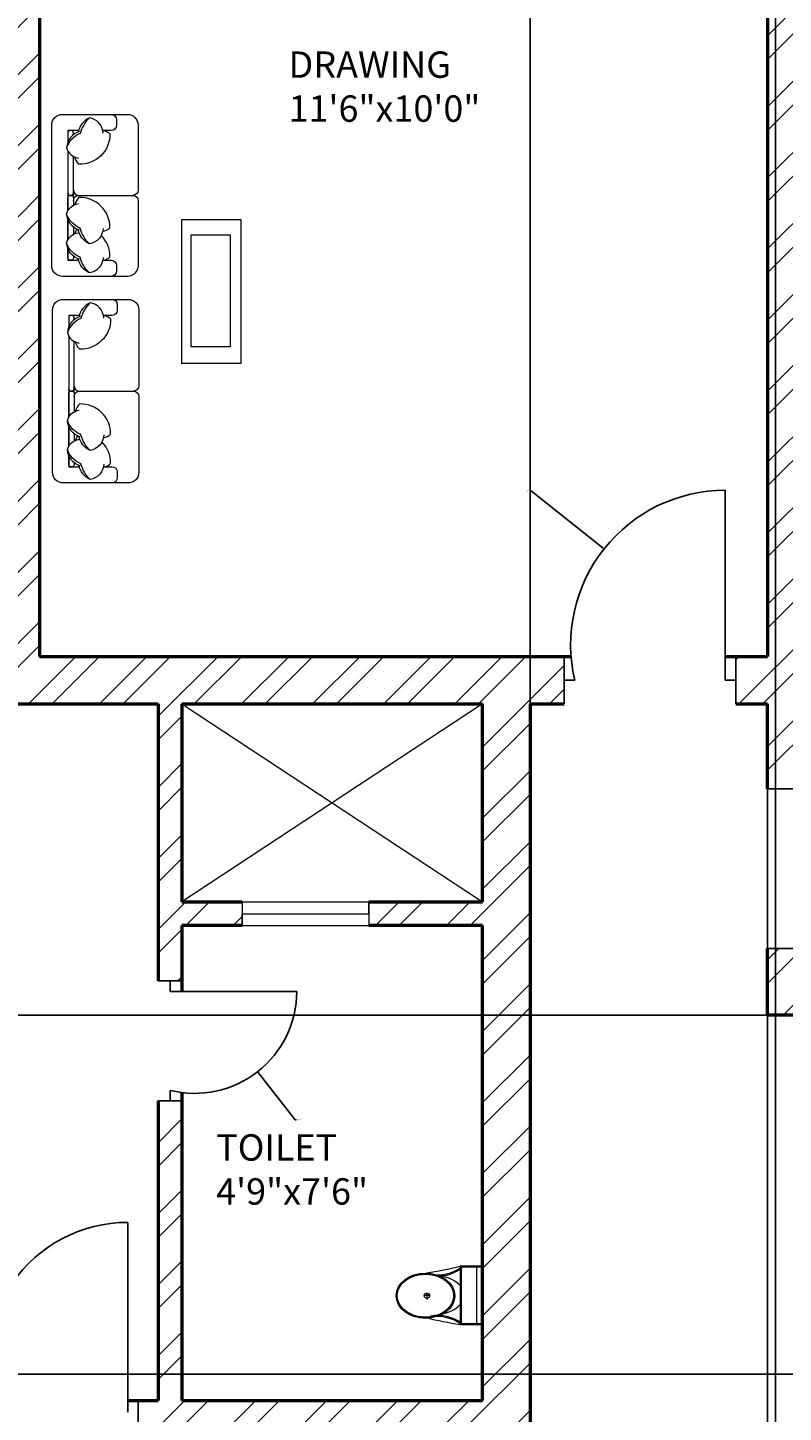
# Model space of a CAD drawing. Units: inches. Extents: x 1896 to 2572, y 1528 to 2474.
# Tile 7 of 10: x 2113 to 2256, y 2033 to 2295. Entities that reach past the tile are written whole.
import ezdxf

# ---------------------------------------------------------------- set-up
doc = ezdxf.new("R2010")
doc.units = ezdxf.units.IN
for name, color, linetype, lineweight in [('A-ANNO-DIMS', 2, 'Continuous', 18), ('A-AREA-IDEN', 7, 'Continuous', 18), ('A-DOOR', 11, 'Continuous', 25), ('A-FLOR-FIXT', 8, 'Continuous', 18), ('A-FLOR-OPEN', 7, 'Continuous', 18), ('A-FURN', 8, 'Continuous', 18), ('A-GLAZ', 131, 'Continuous', 20), ('A-WALL', 7, 'Continuous', 50)]:
    doc.layers.add(name, color=color, linetype=linetype, lineweight=lineweight)
doc.layers.add('A-WALL-PATT', color=215, linetype='Continuous', lineweight=13, true_color=0xa953a0)
doc.styles.get("Standard").update_dxf_attribs({"font": 'arial.ttf'})
doc.dimstyles.get("Standard").update_dxf_attribs({"dimtxt": 0.18, "dimasz": 0.18, "dimexe": 0.18, "dimexo": 0.0625, "dimgap": 0.09, "dimtad": 0, "dimtih": 1, "dimtoh": 1, "dimdec": 4, "dimzin": 0, "dimdsep": 46, "dimtxsty": 'Standard', "dimcen": 0.09, "dimadec": 0, "dimazin": 0, "dimtfac": 1, "dimtdec": 4, "dimtofl": 0, "dimtmove": 0, "dimatfit": 3, "dimfxl": 1, "dimtolj": 1, "dimtzin": 0, "dimarcsym": 0})

# ---------------------------------------------------------------- blocks, each defined once
blk = doc.blocks.new('A$C31115884')
for p, q in [((283, 498), (223, 498)), ((258, 466), (258, 523)), ((0, 200), (0, 0)), ((520, 200), (0, 200)), ((10, 190), (10, 10)), ((510, 190), (10, 190)), ((510, 10), (510, 190)), ((520, 0), (520, 200)), ((510, 54), (0, 54)), ((10, 10), (510, 10)), ((0, 0), (520, 0))]:
    blk.add_line(p, q)
blk.add_circle((256, 496), 23.6)
for centre, radius, start, end in [((2778, -205), 2807, 165.4549, 171.7133), ((3237, 905), 2807, 188.2867, 194.5451), ((-295, 403), 365, 324.2091, 9.3499), ((-295, 403), 375, 324.2091, 9.3499), ((139, 406), 293, 315.8436, 2.6563), ((806, 403), 375, 179.2036, 215.7909), ((806, 403), 365, 170.6501, 215.7909), ((384, 406), 293, 190.2774, 224.1564)]:
    blk.add_arc(centre, radius, start, end)
blk.add_ellipse((256, 510), major_axis=(0, -261), ratio=0.772727)
blk.add_open_spline([(256, 259), (263, 259), (270, 260), (288, 262), (299, 265), (320, 273), (330, 278), (350, 291), (360, 299), (378, 316), (386, 326), (402, 347), (409, 358), (421, 383), (427, 395), (436, 422), (440, 436), (445, 465), (447, 480), (448, 509), (448, 524), (445, 553), (443, 568), (436, 596), (432, 610), (422, 636), (416, 649), (402, 672), (395, 683), (379, 703), (370, 712), (351, 728), (341, 735), (321, 746), (310, 751), (289, 757), (278, 759), (256, 761), (245, 761), (223, 757), (212, 754), (191, 746), (181, 741), (161, 728), (151, 720), (133, 703), (125, 693), (110, 672), (103, 660), (90, 636), (85, 623), (76, 596), (72, 582), (67, 553), (66, 538), (64, 509), (65, 494), (68, 465), (70, 450), (77, 422), (81, 408), (91, 382), (97, 370), (111, 346), (118, 335), (135, 316), (144, 307), (162, 291), (172, 284), (193, 273), (203, 269), (225, 262), (236, 260), (250, 259), (253, 259), (256, 259)], degree=3, knots=[0, 0, 0, 0, 0.110105, 0.110105, 0.285049, 0.285049, 0.459994, 0.459994, 0.634938, 0.634938, 0.809882, 0.809882, 0.984827, 0.984827, 1.159771, 1.159771, 1.334715, 1.334715, 1.50966, 1.50966, 1.684604, 1.684604, 1.859549, 1.859549, 2.034493, 2.034493, 2.209437, 2.209437, 2.384382, 2.384382, 2.559326, 2.559326, 2.73427, 2.73427, 2.909215, 2.909215, 3.084159, 3.084159, 3.259103, 3.259103, 3.434048, 3.434048, 3.608992, 3.608992, 3.783936, 3.783936, 3.958881, 3.958881, 4.133825, 4.133825, 4.30877, 4.30877, 4.483714, 4.483714, 4.658658, 4.658658, 4.833603, 4.833603, 5.008547, 5.008547, 5.183491, 5.183491, 5.358436, 5.358436, 5.53338, 5.53338, 5.708324, 5.708324, 5.883269, 5.883269, 6.058213, 6.058213, 6.233158, 6.233158, 6.283185, 6.283185, 6.283185, 6.283185])
blk = doc.blocks.new('TABLE-COFFEE')
for points in [[(11.21, 0), (0, 0), (0, 27.27), (11.21, 27.27)], [(9.42, 2.87), (2.04, 2.87), (2.04, 24.13), (9.42, 24.13)]]:
    blk.add_lwpolyline(points, close=True)
blk = doc.blocks.new('*D20')
at = {"layer": 'A-ANNO-DIMS', "color": 0, "lineweight": -2, "transparency": 16777216}
for p, q in [((2180.68, 2431.4), (2511.65, 2431.4)), ((2511.47, 2431.22), (2511.47, 2049.83)), ((2511.47, 1668.08), (2511.47, 2049.47)), ((2452.68, 1667.9), (2511.65, 1667.9))]:
    blk.add_line(p, q, dxfattribs=at)
at = {"layer": 'A-ANNO-DIMS', "color": 0, "transparency": 16777216}
for points in [[(2511.44, 2431.22), (2511.5, 2431.22), (2511.47, 2431.4)], [(2511.44, 1668.08), (2511.5, 1668.08), (2511.47, 1667.9)]]:
    blk.add_solid(points, dxfattribs=at)
at = {"layer": 'Defpoints', "color": 0, "transparency": 16777216}
for p in [(2180.62, 2431.4), (2511.47, 2431.4), (2452.62, 1667.9)]:
    blk.add_point(p, dxfattribs=at)
at = {"layer": 'A-ANNO-DIMS', "color": 0, "transparency": 16777216, "insert": (2511.47, 2049.65), "char_height": 0.18, "attachment_point": 5}
blk.add_mtext('\\A1;763.5', dxfattribs=at)
blk = doc.blocks.new('*D30')
at = {"layer": 'A-ANNO-DIMS', "color": 0, "lineweight": -2, "transparency": 16777216}
for p, q in [((2347.56, 2107.9), (1919.59, 2107.9)), ((1919.77, 2107.72), (1919.77, 2074.08)), ((1919.77, 2040.08), (1919.77, 2073.72)), ((2347.56, 2039.9), (1919.59, 2039.9))]:
    blk.add_line(p, q, dxfattribs=at)
at = {"layer": 'A-ANNO-DIMS', "color": 0, "transparency": 16777216}
for points in [[(1919.74, 2107.72), (1919.8, 2107.72), (1919.77, 2107.9)], [(1919.74, 2040.08), (1919.8, 2040.08), (1919.77, 2039.9)]]:
    blk.add_solid(points, dxfattribs=at)
at = {"layer": 'Defpoints', "color": 0, "transparency": 16777216}
for p in [(1919.77, 2107.9), (2347.62, 2107.9), (2347.62, 2039.9)]:
    blk.add_point(p, dxfattribs=at)
at = {"layer": 'A-ANNO-DIMS', "color": 0, "transparency": 16777216, "insert": (1919.77, 2073.9), "char_height": 0.18, "attachment_point": 5}
blk.add_mtext('\\A1;68', dxfattribs=at)
blk = doc.blocks.new('*D33')
at = {"layer": 'A-ANNO-DIMS', "color": 0, "lineweight": -2, "transparency": 16777216}
for p, q in [((2208.12, 2166.84), (2208.12, 1549.1)), ((2253.12, 2166.84), (2253.12, 1549.1)), ((2208.3, 1549.28), (2230.4, 1549.28)), ((2252.94, 1549.28), (2230.85, 1549.28))]:
    blk.add_line(p, q, dxfattribs=at)
at = {"layer": 'A-ANNO-DIMS', "color": 0, "transparency": 16777216}
for points in [[(2208.3, 1549.31), (2208.3, 1549.25), (2208.12, 1549.28)], [(2252.94, 1549.31), (2252.94, 1549.25), (2253.12, 1549.28)]]:
    blk.add_solid(points, dxfattribs=at)
at = {"layer": 'Defpoints', "color": 0, "transparency": 16777216}
for p in [(2208.12, 2166.9), (2253.12, 2166.9), (2253.12, 1549.28)]:
    blk.add_point(p, dxfattribs=at)
at = {"layer": 'A-ANNO-DIMS', "color": 0, "transparency": 16777216, "insert": (2230.62, 1549.28), "char_height": 0.18, "attachment_point": 5}
blk.add_mtext('\\A1;45', dxfattribs=at)
blk = doc.blocks.new('*D34')
at = {"layer": 'A-ANNO-DIMS', "color": 0, "lineweight": -2, "transparency": 16777216}
for p, q in [((2208.12, 1889.96), (2208.12, 2473.93)), ((2208.3, 2473.75), (2231.04, 2473.75)), ((2254.44, 2473.75), (2231.7, 2473.75)), ((2254.62, 1889.96), (2254.62, 2473.93))]:
    blk.add_line(p, q, dxfattribs=at)
at = {"layer": 'A-ANNO-DIMS', "color": 0, "transparency": 16777216}
for points in [[(2208.3, 2473.78), (2208.3, 2473.72), (2208.12, 2473.75)], [(2254.44, 2473.78), (2254.44, 2473.72), (2254.62, 2473.75)]]:
    blk.add_solid(points, dxfattribs=at)
at = {"layer": 'Defpoints', "color": 0, "transparency": 16777216}
for p in [(2254.62, 2473.75), (2208.12, 1889.9), (2254.62, 1889.9)]:
    blk.add_point(p, dxfattribs=at)
at = {"layer": 'A-ANNO-DIMS', "color": 0, "transparency": 16777216, "insert": (2231.37, 2473.75), "char_height": 0.18, "attachment_point": 5}
blk.add_mtext('\\A1;46.5', dxfattribs=at)
blk = doc.blocks.new('*D38')
at = {"layer": 'A-ANNO-DIMS', "color": 0, "lineweight": -2, "transparency": 16777216}
for p, q in [((2208.18, 2207.21), (2208.36, 2207.21)), ((2208.36, 2207.21), (2222, 2196.41)), ((2245.01, 2178.1), (2245.19, 2178.1)), ((2245.1, 2178.01), (2245.1, 2178.19))]:
    blk.add_line(p, q, dxfattribs=at)
at = {"layer": 'A-ANNO-DIMS', "color": 0, "transparency": 16777216}
blk.add_solid([(2222.02, 2196.43), (2221.98, 2196.38), (2222.14, 2196.29)], dxfattribs=at)
at = {"layer": 'Defpoints', "color": 0, "transparency": 16777216}
for p in [(2222.14, 2196.29), (2245.1, 2178.1)]:
    blk.add_point(p, dxfattribs=at)
at = {"layer": 'A-ANNO-DIMS', "color": 0, "transparency": 16777216, "insert": (2207.77, 2207.21), "char_height": 0.18, "attachment_point": 5}
blk.add_mtext('\\A1;R29.3', dxfattribs=at)
blk = doc.blocks.new('*D43')
at = {"layer": 'A-ANNO-DIMS', "color": 0, "lineweight": -2, "transparency": 16777216}
for p, q in [((2096.63, 2066.26), (2096.81, 2066.26)), ((2096.81, 2066.26), (2109.79, 2057.28)), ((2131.74, 2042.03), (2131.92, 2042.03)), ((2131.83, 2041.94), (2131.83, 2042.12))]:
    blk.add_line(p, q, dxfattribs=at)
at = {"layer": 'A-ANNO-DIMS', "color": 0, "transparency": 16777216}
blk.add_solid([(2109.81, 2057.3), (2109.78, 2057.25), (2109.94, 2057.18)], dxfattribs=at)
at = {"layer": 'Defpoints', "color": 0, "transparency": 16777216}
for p in [(2109.94, 2057.18), (2131.83, 2042.03)]:
    blk.add_point(p, dxfattribs=at)
at = {"layer": 'A-ANNO-DIMS', "color": 0, "transparency": 16777216, "insert": (2096.15, 2066.26), "char_height": 0.18, "attachment_point": 5}
blk.add_mtext('\\A1;R26.62', dxfattribs=at)
blk = doc.blocks.new('*D47')
at = {"layer": 'A-ANNO-DIMS', "color": 0, "lineweight": -2, "transparency": 16777216}
for p, q in [((2144.54, 2112.33), (2144.54, 2112.51)), ((2144.45, 2112.42), (2144.63, 2112.42)), ((2163.59, 2088.06), (2156.56, 2097.05)), ((2163.77, 2088.06), (2163.59, 2088.06))]:
    blk.add_line(p, q, dxfattribs=at)
at = {"layer": 'A-ANNO-DIMS', "color": 0, "transparency": 16777216}
blk.add_solid([(2156.58, 2097.07), (2156.53, 2097.03), (2156.45, 2097.19)], dxfattribs=at)
at = {"layer": 'Defpoints', "color": 0, "transparency": 16777216}
for p in [(2144.54, 2112.42), (2156.45, 2097.19)]:
    blk.add_point(p, dxfattribs=at)
at = {"layer": 'A-ANNO-DIMS', "color": 0, "transparency": 16777216, "insert": (2164.25, 2088.06), "char_height": 0.18, "attachment_point": 5}
blk.add_mtext('\\A1;R19.33', dxfattribs=at)

msp = doc.modelspace()

# ---------------------------------------------------------------- hatches: boundary and pattern name
at = {"layer": 'A-WALL-PATT'}
h = msp.add_hatch(dxfattribs=at)
h.set_pattern_fill('ANSI32', color=256)
h.paths.add_polyline_path([(2071.6224, 2382.3979), (2071.6224, 2422.3979), (2110.6224, 2422.3979), (2110.6224, 2382.3979), (2110.6224, 2357.5961), (2119.6224, 2357.5961), (2119.6224, 2422.3979), (2171.6224, 2422.3979), (2171.6224, 2373.3979), (2193.5093, 2373.3979), (2193.5093, 2377.8979), (2193.5093, 2382.3979), (2180.6224, 2382.3979), (2180.6224, 2431.3979), (2171.6224, 2431.3979), (2119.6224, 2431.3979), (2110.6224, 2431.3979), (2062.6224, 2431.3979), (2062.6224, 2422.3979), (2062.6224, 2382.3979), (1978.6224, 2382.3979), (1978.6224, 2313.0337), (1987.6224, 2313.0337), (1987.6224, 2373.3979), (2062.6224, 2373.3979), (2067.1224, 2373.3979), (2067.1224, 2353.7982), (2071.6224, 2353.8883)])
h.paths.add_polyline_path([(2287.4624, 2382.3979), (2229.5093, 2382.3979), (2229.5093, 2373.3979), (2253.1224, 2373.3979), (2253.1224, 2175.8979), (2247.1039, 2175.8979), (2247.1039, 2166.8979), (2253.1224, 2166.8979), (2253.1224, 2150.8283), (2262.1224, 2150.8283), (2262.1224, 2166.8979), (2262.1224, 2236.8979), (2349.0731, 2236.8979), (2349.0731, 2239.1479), (2349.0731, 2241.3979), (2262.1224, 2241.3979), (2262.1224, 2373.3979), (2287.4624, 2373.3979)])
h.paths.add_polyline_path([(2452.6224, 2382.3979), (2347.4624, 2382.3979), (2347.4624, 2373.3979), (2382.1224, 2373.3979), (2382.1224, 2334.0335), (2386.6224, 2334.0335), (2386.6224, 2373.3979), (2443.6224, 2373.3979), (2443.6224, 2316.2056), (2452.6224, 2316.2056)])
h.paths.add_polyline_path([(2452.6224, 2292.2056), (2448.1224, 2292.2056), (2443.6224, 2292.2056), (2443.6224, 2292.0047), (2443.6224, 2280.9372), (2443.6224, 2268.3979), (2386.6224, 2268.3979), (2386.6224, 2312.4044), (2384.3724, 2312.4044), (2382.1224, 2312.4044), (2382.1224, 2241.3979), (2379.1336, 2241.3979), (2379.1336, 2236.8979), (2386.6224, 2236.8979), (2386.6224, 2263.8979), (2443.6224, 2263.8979), (2443.6224, 2248.8449), (2452.6224, 2248.8449)])
h.paths.add_polyline_path([(2364.1285, 2116.8979), (2262.1224, 2116.8979), (2262.1224, 2120.5401), (2257.6224, 2120.5401), (2253.1224, 2120.5401), (2253.1224, 2107.8979), (2262.1224, 2107.8979), (2269.354, 2107.8979), (2269.354, 2094.0702), (2278.354, 2094.0702), (2278.354, 2107.8979), (2347.6224, 2107.8979), (2347.6224, 2039.8979), (2278.354, 2039.8979), (2278.354, 2054.7605), (2269.354, 2054.7605), (2269.354, 2030.8979), (2278.354, 2030.8979), (2443.6224, 2030.8979), (2443.6224, 2015.198), (2452.6224, 2015.198), (2452.6224, 2030.8979), (2464.6224, 2030.8979), (2469.1224, 2030.8979), (2469.1224, 2117.0352), (2452.6767, 2116.9466), (2452.6285, 2125.8979), (2452.6224, 2125.8979), (2452.6224, 2212.8449), (2443.6224, 2212.8449), (2443.6224, 2116.8979), (2385.832, 2116.8979), (2385.832, 2112.3979), (2385.832, 2107.8979), (2464.6224, 2107.8979), (2464.6224, 2039.8979), (2443.6224, 2039.8979), (2356.6224, 2039.8979), (2356.6224, 2107.8979), (2364.1285, 2107.8979)])
h.paths.add_polyline_path([(2452.6224, 1967.198), (2443.6224, 1967.198), (2443.6224, 1955.8979), (2259.1224, 1955.8979), (2254.6224, 1955.8979), (2254.6224, 1941.6358), (2263.6224, 1941.6358), (2263.6224, 1946.8979), (2379.1224, 1946.8979), (2379.1224, 1913.0204), (2383.6224, 1913.0204), (2383.6224, 1946.8979), (2443.6224, 1946.8979), (2443.6224, 1930.729), (2452.6224, 1930.729)])
h.paths.add_polyline_path([(2469.1224, 1871.8979), (2464.6224, 1871.8979), (2452.6224, 1871.8979), (2452.6224, 1894.729), (2443.6224, 1894.729), (2443.6224, 1871.8979), (2388.1304, 1871.8979), (2388.1304, 1867.3979), (2443.6224, 1867.3979), (2464.6224, 1867.3979), (2464.6224, 1817.8979), (2443.6224, 1817.8979), (2388.1304, 1817.8979), (2388.1304, 1815.6479), (2388.1304, 1813.3979), (2391.1224, 1813.3979), (2391.1224, 1747.8899), (2395.6224, 1747.8899), (2395.6224, 1813.3979), (2443.6224, 1813.3979), (2443.6224, 1781.4434), (2452.6224, 1781.4434), (2452.6224, 1813.3979), (2464.6224, 1813.3979), (2469.1224, 1813.3979)])
h.paths.add_polyline_path([(2263.6224, 1910.9737), (2259.1224, 1910.9737), (2254.6224, 1910.9737), (2254.6224, 1889.8979), (2251.2778, 1889.8979), (2251.2778, 1880.8979), (2254.6224, 1880.8979), (2254.6224, 1817.8979), (2254.6224, 1754.8979), (2254.6224, 1693.3979), (2254.6224, 1684.3979), (2254.6224, 1672.3979), (2200.6224, 1672.3979), (2200.6224, 1684.3979), (2200.6224, 1693.3979), (2200.6224, 1754.8979), (2196.1224, 1754.8979), (2196.1224, 1693.3979), (2150.0488, 1693.3979), (2150.0488, 1684.3979), (2196.1224, 1684.3979), (2196.1224, 1672.3979), (2196.1224, 1667.8979), (2254.6224, 1667.8979), (2259.1224, 1667.8979), (2259.1224, 1693.3979), (2259.1224, 1813.3979), (2353.6224, 1813.3979), (2353.6224, 1815.6479), (2353.6224, 1817.8979), (2263.6224, 1817.8979)])
h.paths.add_polyline_path([(2391.1224, 1693.3979), (2345.6981, 1693.3979), (2345.6981, 1684.3979), (2391.1224, 1684.3979)])
h.paths.add_polyline_path([(2285.6981, 1693.3979), (2259.1224, 1693.3979), (2259.1224, 1684.3979), (2285.6981, 1684.3979), (2285.6981, 1688.8979)], flags=17)
h.paths.add_polyline_path([(2452.6224, 1757.4434), (2448.1224, 1757.4434), (2443.6224, 1757.4434), (2443.6224, 1726.3979), (2395.6224, 1726.3979), (2395.6224, 1728.6572), (2393.3724, 1728.6572), (2391.1224, 1728.6572), (2391.1224, 1717.6723), (2395.6224, 1717.6723), (2395.6224, 1721.8979), (2443.6224, 1721.8979), (2443.6224, 1714.8), (2452.6224, 1714.8)])
h.paths.add_polyline_path([(2452.6224, 1684.3979), (2452.6224, 1690.8), (2443.6224, 1690.8), (2443.6224, 1679.8979), (2443.6224, 1672.3979), (2395.6224, 1672.3979), (2395.6224, 1695.6708), (2391.1224, 1695.5986), (2391.1224, 1672.3979), (2391.1224, 1667.8979), (2452.6224, 1667.8979)])
h.paths.add_polyline_path([(1987.6224, 1880.8979), (2068.6224, 1880.8979), (2125.6224, 1880.8979), (2125.6224, 1788.8466), (2130.1224, 1788.8466), (2130.1224, 1880.8979), (2216.1958, 1880.8979), (2216.1958, 1885.3979), (2216.1958, 1889.8979), (2208.1224, 1889.8979), (2208.1224, 1996.3717), (2203.6224, 1996.3717), (2199.1224, 1996.3717), (2199.1224, 1889.8979), (2073.1224, 1889.8979), (2073.1224, 1917.1874), (2068.6224, 1917.1874), (2068.6224, 1889.8979), (1987.6224, 1889.8979), (1987.6224, 1912.4976), (1978.6224, 1912.4976), (1978.6224, 1805.5193), (1987.6224, 1805.5193)])
h.paths.add_polyline_path([(2019.9303, 1754.8979), (1987.6224, 1754.8979), (1966.6224, 1754.8979), (1966.6224, 1801.0193), (1987.6224, 1801.0193), (1987.6224, 1805.5193), (1962.1224, 1805.5193), (1962.1224, 1750.3979), (1966.6224, 1750.3979), (1978.6224, 1750.3979), (1987.6224, 1750.3979), (2019.9303, 1750.3979)])
h.paths.add_polyline_path([(2135.5566, 1754.8979), (2130.1224, 1754.8979), (2130.1224, 1758.052), (2127.8724, 1758.052), (2125.6224, 1758.052), (2125.6224, 1754.8979), (2068.6224, 1754.8979), (2043.2292, 1754.8979), (2043.2292, 1750.3979), (2068.6224, 1750.3979), (2098.6224, 1750.3979), (2098.6224, 1693.3979), (2068.6224, 1693.3979), (1987.6224, 1693.3979), (1987.6224, 1707.3003), (1983.1224, 1707.3003), (1978.6224, 1707.3003), (1978.6224, 1684.3979), (2068.6224, 1684.3979), (2126.0488, 1684.3979), (2126.0488, 1688.8979), (2126.0488, 1693.3979), (2103.1224, 1693.3979), (2103.1224, 1750.3979), (2130.1224, 1750.3979), (2135.5566, 1750.3979)])
h.paths.add_polyline_path([(1987.6224, 1750.3979), (1978.6224, 1750.3979), (1978.6224, 1731.3003), (1987.6224, 1731.3003)], flags=0)
h.paths.add_polyline_path([(1987.6224, 1973.8979), (2068.6224, 1973.8979), (2073.1224, 1973.8979), (2073.1224, 1978.3979), (1971.1224, 1978.3979), (1971.1224, 2030.3979), (1978.6224, 2030.3979), (1987.6224, 2030.3979), (2104.9199, 2030.3979), (2104.9199, 2032.6479), (2104.9199, 2034.8979), (1987.6224, 2034.8979), (1971.1224, 2034.8979), (1971.1224, 2085.8979), (2003.6464, 2085.8979), (2003.6464, 2090.3979), (1987.6224, 2090.3979), (1987.6224, 2166.8979), (2115.1224, 2166.8979), (2137.6224, 2166.8979), (2137.6224, 2114.4229), (2142.1224, 2114.4229), (2142.1224, 2124.8979), (2153.5306, 2124.8979), (2153.5306, 2127.1479), (2153.5306, 2129.3979), (2142.1224, 2129.3979), (2142.1224, 2166.8979), (2199.1224, 2166.8979), (2199.1224, 2129.3979), (2177.5306, 2129.3979), (2177.5306, 2124.8979), (2199.1224, 2124.8979), (2199.1224, 2034.8979), (2142.1224, 2034.8979), (2142.1224, 2091.6671), (2139.8724, 2091.6671), (2137.6224, 2091.6671), (2137.6224, 2034.8979), (2133.8326, 2034.8979), (2133.8326, 2030.3979), (2137.6224, 2030.3979), (2142.1224, 2030.3979), (2199.1224, 2030.3979), (2199.1224, 2024.2654), (2208.1224, 2024.2654), (2208.1224, 2030.3979), (2208.1224, 2166.8979), (2214.5775, 2166.8979), (2214.5775, 2171.3979), (2214.5775, 2175.8979), (2115.1224, 2175.8979), (2115.1224, 2329.9154), (2112.4137, 2329.9154), (2110.6224, 2329.9154), (2110.6224, 2175.8979), (2082.1224, 2175.8979), (2082.1224, 2202.6443), (2079.8724, 2202.6443), (2077.6224, 2202.6443), (2077.6224, 2175.8979), (1987.6224, 2175.8979), (1987.6224, 2191.3531), (1983.1224, 2191.3531), (1978.6224, 2191.3531), (1978.6224, 2090.3979), (1966.6224, 2090.3979), (1966.6224, 2085.8979), (1966.6224, 2030.3979), (1966.6224, 1973.8979), (1978.6224, 1973.8979), (1978.6224, 1948.4976), (1983.1224, 1948.4976), (1987.6224, 1948.4976)])
h.paths.add_polyline_path([(1987.6224, 2253.0337), (1983.1224, 2253.0337), (1978.6224, 2253.0337), (1978.6224, 2215.3531), (1987.6224, 2215.3531), (1987.6224, 2224.8979), (2077.6224, 2224.8979), (2077.6224, 2221.9854), (2082.1224, 2221.9854), (2082.1224, 2229.3979), (1987.6224, 2229.3979)], flags=17)
h.paths.add_polyline_path([(2220.5047, 1978.7278), (2253.7278, 1978.7278), (2253.7278, 1997.3851), (2220.5047, 1997.3851)], flags=9)
h.paths.add_polyline_path([(2303.6746, 2064.9806), (2320.5334, 2064.9806), (2320.5334, 2075.2842), (2303.6746, 2075.2842)], flags=25)

# ---------------------------------------------------------------- linework, layer by layer
at = {"layer": 'A-DOOR'}
for p, q in [((2245.1039, 2171.3979), (2245.1039, 2207.3979)), ((2214.5775, 2175.8979), (2214.5775, 2166.8979)), ((2247.1039, 2175.8979), (2247.1039, 2166.8979)), ((2214.5775, 2166.8979), (2214.5775, 2171.3979)), ((2214.5775, 2171.3979), (2216.5775, 2171.3979)), ((2247.1039, 2171.3979), (2245.1039, 2171.3979)), ((2247.1039, 2166.8979), (2247.1039, 2171.3979)), ((2253.1224, 2150.8283), (2262.1224, 2150.8283)), ((2253.1224, 2120.5401), (2262.1224, 2120.5401)), ((2137.6224, 2114.4229), (2142.1224, 2114.4229)), ((2142.1224, 2114.4229), (2139.8724, 2114.4229)), ((2139.8724, 2114.4229), (2139.8724, 2112.4229)), ((2139.8724, 2112.4229), (2163.8724, 2112.4229)), ((2137.6224, 2091.6671), (2142.1224, 2091.6671)), ((2139.8724, 2091.6671), (2139.8724, 2093.6671)), ((2142.1224, 2091.6671), (2139.8724, 2091.6671)), ((2131.8326, 2032.6479), (2131.8326, 2068.6479)), ((2133.8326, 2034.8979), (2133.8326, 2030.3979))]:
    msp.add_line(p, q, dxfattribs=at)
for centre, radius, start, end in [((2245.1039, 2178.0957), 29.3022, 90, 193.213291), ((2144.5436, 2112.4229), 19.3288, 256.014793, 0), ((2131.8326, 2042.0278), 26.6201, 90, 200.631887)]:
    msp.add_arc(centre, radius, start, end, dxfattribs=at)
at = {"layer": 'A-FLOR-OPEN'}
for p, q in [((2199.1224, 2166.8979), (2142.1224, 2129.3979)), ((2142.1224, 2166.8979), (2199.1224, 2129.3979))]:
    msp.add_line(p, q, dxfattribs=at)
at = {"layer": 'A-FURN', "ltscale": 0.03}
for points in [[(2133.8117, 2264.3035, -0.41421356), (2132.7883, 2263.2801, -0.41421356), (2133.8117, 2262.2567), (2133.8117, 2249.9758, -0.41421356), (2131.7649, 2247.929), (2119.484, 2247.929, -0.41421356), (2117.4371, 2249.9758), (2117.4371, 2276.5844, -0.41421356), (2119.484, 2278.6312), (2131.7649, 2278.6312, -0.41421356), (2133.8117, 2276.5844), (2133.8117, 2264.3035, -0.41421356), (2132.7883, 2263.2801, -0.41421356), (2133.8117, 2262.2567)], [(2133.9492, 2227.2045, -0.41421356), (2132.9258, 2226.181, -0.41421356), (2133.9492, 2225.1576), (2133.9492, 2210.8299, -0.41421356), (2131.9023, 2208.7831), (2119.6215, 2208.7831, -0.41421356), (2117.5746, 2210.8299), (2117.5746, 2241.5322, -0.41421356), (2119.6215, 2243.579), (2131.9023, 2243.579, -0.41421356), (2133.9492, 2241.5322), (2133.9492, 2227.2045, -0.41421356), (2132.9258, 2226.181, -0.41421356), (2133.9492, 2225.1576)]]:
    msp.add_lwpolyline(points, format="xyb", dxfattribs=at)
at = {"layer": 'A-FURN'}
for points in [[(2124.5913, 2277.9799, 0.14772988), (2122.8325, 2274.9888, 0.21334276), (2120.2529, 2272.3495, 0.17866181)], [(2127.1709, 2275.0474, 0.35677236), (2124.5913, 2277.9799, 0.24954205), (2122.4655, 2275.3228, -9.61688035)], [(2128.6946, 2278.6312, -0.41421356), (2129.718, 2277.6078), (2129.718, 2276.5844, -0.41421356), (2128.6946, 2275.561), (2127.109, 2275.561)], [(2122.6923, 2275.402, 0.30666349), (2120.2529, 2272.3495, 0.30632997), (2122.4807, 2270.3554, -0.87284716)], [(2121.5308, 2274.78), (2121.5308, 2275.1516, 0.41421356), (2121.1214, 2275.561), (2120.9167, 2275.561, 0.41421356), (2120.5074, 2275.1516)], [(2120.5074, 2275.1516), (2120.5074, 2273.408, 0.41421356)], [(2127.1085, 2275.5632, -0.16554063), (2128.4607, 2274.9301, -0.42598917), (2122.598, 2269.1825, -0.12152332), (2121.7899, 2270.5468, 7.11546429)], [(2120.5074, 2271.7055), (2120.5074, 2263.6895, 0.41421356), (2120.9167, 2263.2801), (2121.1214, 2263.2801, 0.41421356), (2121.5308, 2263.6895), (2121.5308, 2270.6749, 0.41421356)], [(2120.5074, 2260.3678), (2120.5074, 2262.8707, -0.41421356), (2120.9167, 2263.2801), (2121.1214, 2263.2801, -0.41421356), (2121.5308, 2262.8707), (2121.5308, 2261.3983, -0.41421356)], [(2121.5308, 2264.3035, 0.41421356), (2122.5542, 2263.2801)], [(2121.5308, 2264.3035, 0.41421356), (2122.5542, 2263.2801), (2132.7883, 2263.2801, 0.41421356)], [(2121.5308, 2262.2567, -0.41421356), (2122.5542, 2263.2801)], [(2121.5308, 2262.2567, -0.41421356), (2122.5542, 2263.2801), (2132.7883, 2263.2801, -0.41421356)], [(2127.1085, 2256.51, 0.16554063), (2128.4607, 2257.1432, 0.42598917), (2122.598, 2262.8908, 0.12152332), (2121.7899, 2261.5264, -7.11546429)], [(2122.6923, 2256.6713, -0.30666349), (2120.2529, 2259.7237, -0.30632997), (2122.4807, 2261.7178, 0.87284716)], [(2124.5913, 2254.0934, -0.14772988), (2122.8325, 2257.0845, -0.21334276), (2120.2529, 2259.7237, -0.17866181)], [(2120.5074, 2254.8548), (2120.5074, 2258.6652, -0.41421356)], [(2121.5308, 2257.2932), (2121.5308, 2255.8853, -0.41421356)], [(2122.19, 2256.8714, 0.07186538), (2121.7899, 2256.0134, -7.11546429)], [(2127.1709, 2257.0259, -0.35677236), (2124.5913, 2254.0934, -0.24954205), (2122.4655, 2256.7505, 9.61688035)], [(2122.6923, 2251.1582, -0.30666349), (2120.2529, 2254.2107, -0.30632997), (2122.4807, 2256.2048, 0.87284716)], [(2124.5913, 2248.5803, -0.14772988), (2122.8325, 2251.5714, -0.21334276), (2120.2529, 2254.2107, -0.17866181)], [(2127.1085, 2250.997, 0.16554063), (2128.4607, 2251.6301, 0.20023115), (2126.8139, 2255.6926, 0.12152332)], [(2120.5074, 2251.4086), (2120.5074, 2253.1522, -0.41421356)], [(2120.5074, 2253.1522), (2120.5074, 2250.9992), (2122.5186, 2250.9992, -0.41421356)], [(2121.5308, 2251.7802), (2121.5308, 2251.4086, -0.41421356), (2121.1214, 2250.9992), (2120.9167, 2250.9992, -0.41421356), (2120.5074, 2251.4086)], [(2127.1709, 2251.5128, -0.35677236), (2124.5913, 2248.5803, -0.24954205), (2122.4655, 2251.2374, 9.61688035)], [(2127.109, 2250.9992), (2128.6946, 2250.9992, -0.41421356), (2129.718, 2249.9758), (2129.718, 2248.9524, -0.41421356), (2128.6946, 2247.929)], [(2124.7288, 2242.9276, 0.14772988), (2122.97, 2239.9365, 0.21334276), (2120.3904, 2237.2973, 0.17866181)], [(2127.3084, 2239.9952, 0.35677236), (2124.7288, 2242.9276, 0.24954205), (2122.603, 2240.2706, -9.61688035)], [(2128.8321, 2243.579, -0.41421356), (2129.8555, 2242.5556), (2129.8555, 2241.5322, -0.41421356), (2128.8321, 2240.5088), (2127.2465, 2240.5088)], [(2122.8298, 2240.3497, 0.30666349), (2120.3904, 2237.2973, 0.30632997), (2122.6182, 2235.3032, -0.87284716)], [(2121.6683, 2239.7278), (2121.6683, 2240.0994, 0.41421356), (2121.2589, 2240.5088), (2121.0542, 2240.5088, 0.41421356), (2120.6449, 2240.0994)], [(2120.6449, 2240.0994), (2120.6449, 2238.3558, 0.41421356)], [(2127.246, 2240.511, -0.16554063), (2128.5982, 2239.8779, -0.42598917), (2122.7355, 2234.1302, -0.12152332), (2121.9274, 2235.4946, 7.11546429)], [(2120.6449, 2236.6532), (2120.6449, 2226.5904, 0.41421356), (2121.0542, 2226.181), (2121.2589, 2226.181, 0.41421356), (2121.6683, 2226.5904), (2121.6683, 2235.6227, 0.41421356)], [(2120.6449, 2221.2219), (2120.6449, 2225.7717, -0.41421356), (2121.0542, 2226.181), (2121.2589, 2226.181, -0.41421356), (2121.6683, 2225.7717), (2121.6683, 2222.2524, -0.41421356)], [(2121.6683, 2227.2045, 0.41421356), (2122.6917, 2226.181)], [(2121.6683, 2227.2045, 0.41421356), (2122.6917, 2226.181), (2132.9258, 2226.181, 0.41421356)], [(2121.6683, 2225.1576, -0.41421356), (2122.6917, 2226.181)], [(2121.6683, 2225.1576, -0.41421356), (2122.6917, 2226.181), (2132.9258, 2226.181, -0.41421356)], [(2127.246, 2217.3642, 0.16554063), (2128.5982, 2217.9973, 0.42598917), (2122.7355, 2223.7449, 0.12152332), (2121.9274, 2222.3806, -7.11546429)], [(2122.8298, 2217.5254, -0.30666349), (2120.3904, 2220.5779, -0.30632997), (2122.6182, 2222.5719, 0.87284716)], [(2124.7288, 2214.9475, -0.14772988), (2122.97, 2217.9386, -0.21334276), (2120.3904, 2220.5779, -0.17866181)], [(2120.6449, 2215.7089), (2120.6449, 2219.5194, -0.41421356)], [(2121.6683, 2218.1474), (2121.6683, 2216.7394, -0.41421356)], [(2122.3275, 2217.7255, 0.07186538), (2121.9274, 2216.8675, -7.11546429)], [(2127.3084, 2217.88, -0.35677236), (2124.7288, 2214.9475, -0.24954205), (2122.603, 2217.6046, 9.61688035)], [(2122.8298, 2212.0123, -0.30666349), (2120.3904, 2215.0648, -0.30632997), (2122.6182, 2217.0589, 0.87284716)], [(2124.7288, 2209.4344, -0.14772988), (2122.97, 2212.4256, -0.21334276), (2120.3904, 2215.0648, -0.17866181)], [(2127.246, 2211.8511, 0.16554063), (2128.5982, 2212.4842, 0.20023115), (2126.9514, 2216.5468, 0.12152332)], [(2120.6449, 2214.0063), (2120.6449, 2211.8533), (2122.6561, 2211.8533, -0.41421356)], [(2120.6449, 2212.2627), (2120.6449, 2214.0063, -0.41421356)], [(2121.6683, 2212.6343), (2121.6683, 2212.2627, -0.41421356), (2121.2589, 2211.8533), (2121.0542, 2211.8533, -0.41421356), (2120.6449, 2212.2627)], [(2127.3084, 2212.3669, -0.35677236), (2124.7288, 2209.4344, -0.24954205), (2122.603, 2212.0915, 9.61688035)], [(2127.2465, 2211.8533), (2128.8321, 2211.8533, -0.41421356), (2129.8555, 2210.8299), (2129.8555, 2209.8065, -0.41421356), (2128.8321, 2208.7831)]]:
    msp.add_lwpolyline(points, format="xyb", dxfattribs=at)
for points in [[(2122.5186, 2275.561), (2120.5074, 2275.561), (2120.5074, 2273.408)], [(2120.5074, 2271.7055), (2120.5074, 2260.3678)], [(2120.5074, 2258.6652), (2120.5074, 2254.8548)], [(2122.6561, 2240.5088), (2120.6449, 2240.5088), (2120.6449, 2238.3558)], [(2120.6449, 2236.6532), (2120.6449, 2221.2219)], [(2120.6449, 2219.5194), (2120.6449, 2215.7089)]]:
    msp.add_lwpolyline(points, dxfattribs=at)
for points in [[(2120.5074, 2263.6895), (2120.5074, 2262.8707, -0.41421356), (2120.9167, 2263.2801), (2121.1214, 2263.2801, -0.41421356), (2121.5308, 2262.8707), (2121.5308, 2263.6895, -0.41421356), (2121.1214, 2263.2801), (2120.9167, 2263.2801, -0.41421356)], [(2120.6449, 2226.5904), (2120.6449, 2225.7717, -0.41421356), (2121.0542, 2226.181), (2121.2589, 2226.181, -0.41421356), (2121.6683, 2225.7717), (2121.6683, 2226.5904, -0.41421356), (2121.2589, 2226.181), (2121.0542, 2226.181, -0.41421356)]]:
    msp.add_lwpolyline(points, format="xyb", close=True, dxfattribs=at)
at = {"layer": 'A-GLAZ'}
for p, q in [((2153.5306, 2129.3979), (2153.5306, 2124.8979)), ((2153.5306, 2129.3979), (2177.5306, 2129.3979)), ((2177.5306, 2127.1479), (2177.5306, 2129.3979)), ((2177.5306, 2129.3979), (2177.5306, 2124.8979)), ((2153.5306, 2124.8979), (2153.5306, 2127.1479)), ((2153.5306, 2127.1479), (2177.5306, 2127.1479)), ((2153.5306, 2124.8979), (2177.5306, 2124.8979))]:
    msp.add_line(p, q, dxfattribs=at)
at = {"layer": 'A-WALL'}
for p, q in [((2253.1224, 2373.3979), (2253.1224, 2175.8979)), ((2115.1224, 2329.9154), (2115.1224, 2175.8979)), ((2115.1224, 2175.8979), (2215.8843, 2175.8979)), ((2245.1039, 2175.8979), (2253.1224, 2175.8979)), ((1987.6224, 2166.8979), (2115.1224, 2166.8979)), ((2115.1224, 2166.8979), (2137.6224, 2166.8979)), ((2137.6224, 2166.8979), (2137.6224, 2114.4229)), ((2142.1224, 2166.8979), (2142.1224, 2129.3979)), ((2142.1224, 2166.8979), (2199.1224, 2166.8979)), ((2199.1224, 2129.3979), (2199.1224, 2166.8979)), ((2208.1224, 2166.8979), (2208.1224, 2030.3979)), ((2208.1224, 2166.8979), (2214.5775, 2166.8979)), ((2247.1039, 2166.8979), (2253.1224, 2166.8979)), ((2253.1224, 2150.8283), (2253.1224, 2166.8979)), ((2142.1224, 2129.3979), (2153.5306, 2129.3979)), ((2177.5306, 2129.3979), (2199.1224, 2129.3979)), ((2142.1224, 2124.8979), (2142.1224, 2112.4229)), ((2153.5306, 2124.8979), (2142.1224, 2124.8979)), ((2199.1224, 2124.8979), (2177.5306, 2124.8979)), ((2199.1224, 2034.8979), (2199.1224, 2124.8979)), ((2199.1224, 2034.8979), (2199.1224, 2124.8979)), ((2253.1224, 2107.8979), (2253.1224, 2120.5401)), ((2262.1224, 2107.8979), (2253.1224, 2107.8979)), ((2137.6224, 2091.6671), (2137.6224, 2034.8979)), ((2142.1224, 2093.2464), (2142.1224, 2034.8979)), ((2131.8326, 2034.8979), (2137.6224, 2034.8979)), ((2142.1224, 2034.8979), (2199.1224, 2034.8979))]:
    msp.add_line(p, q, dxfattribs=at)

# ---------------------------------------------------------------- block references
at = {"layer": 'A-FLOR-FIXT', "xscale": 0.021283599635143, "yscale": 0.021283599635143, "zscale": 0.021283599635143, "rotation": 89.99999999999999}
msp.add_blockref('A$C31115884', (2199.1224, 2049.293), dxfattribs=at)
at = {"layer": 'A-FURN', "rotation": 180}
msp.add_blockref('TABLE-COFFEE', (2153.3034, 2258.6912), dxfattribs=at)

# ---------------------------------------------------------------- texts
at = {"layer": 'A-AREA-IDEN', "char_height": 5, "attachment_point": 1}
for s, width, insert in [('DRAWING\\P11\'6"x10\'0"', 151.261843, (2162.326, 2290.56)), ('TOILET\\P4\'9"x7\'6"', 111.229772, (2148.6027, 2085.3419))]:
    msp.add_mtext_dynamic_manual_height_columns(s, width=width, gutter_width=12.5, heights=[0], dxfattribs=dict(at, insert=insert))

# ---------------------------------------------------------------- dimensions: what is measured, and where the dimension line sits
at = {"layer": 'A-ANNO-DIMS'}
for base, p1, p2, override, picture, middle in [((2254.6224, 2473.7479), (2208.1224, 1889.8979), (2254.6224, 1889.8979), {"dimdec": 1, "dimlfac": 1, "dimrnd": 0, "dimzin": 0, "dimdsep": 46, "dimlunit": 2}, '*D34', (2231.3724, 2473.7479)), ((2253.1224, 1549.2803), (2208.1224, 2166.8979), (2253.1224, 2166.8979), {"dimdec": 0, "dimlfac": 1, "dimrnd": 0, "dimzin": 0, "dimdsep": 46, "dimlunit": 2}, '*D33', (2230.6224, 1549.2803))]:
    dim = msp.add_linear_dim(base=base, p1=p1, p2=p2, dimstyle='Standard', override=override, dxfattribs=at)
    dim.commit()
    dim.dimension.update_dxf_attribs({"geometry": picture, "text_midpoint": middle})
for base, p1, p2, override, picture, middle in [((2511.4724, 2431.3979), (2452.6224, 1667.8979), (2180.6224, 2431.3979), {"dimdec": 1, "dimlfac": 1, "dimrnd": 0, "dimzin": 0, "dimdsep": 46, "dimlunit": 2}, '*D20', (2511.4724, 2049.6479)), ((1919.7724, 2107.8979), (2347.6224, 2039.8979), (2347.6224, 2107.8979), {"dimdec": 0, "dimlfac": 1, "dimrnd": 0, "dimzin": 0, "dimdsep": 46, "dimlunit": 2}, '*D30', (1919.7724, 2073.8979))]:
    dim = msp.add_linear_dim(base=base, p1=p1, p2=p2, angle=90, dimstyle='Standard', override=override, dxfattribs=at)
    dim.commit()
    dim.dimension.update_dxf_attribs({"geometry": picture, "text_midpoint": middle})
for center, mpoint, override, picture, middle in [((2245.1039, 2178.0957), (2222.1379, 2196.2941), {"dimdec": 1, "dimlfac": 1, "dimrnd": 0, "dimzin": 0, "dimdsep": 46, "dimlunit": 2}, '*D38', (2207.7684, 2207.2131)), ((2144.5436, 2112.4229), (2156.4458, 2097.1933), {"dimdec": 2, "dimlfac": 1, "dimrnd": 0, "dimzin": 0, "dimdsep": 46, "dimlunit": 2}, '*D47', (2164.2469, 2088.0555)), ((2131.8326, 2042.0278), (2109.9429, 2057.176), {"dimdec": 2, "dimlfac": 1, "dimrnd": 0, "dimzin": 0, "dimdsep": 46, "dimlunit": 2}, '*D43', (2096.1502, 2066.265))]:
    dim = msp.add_radius_dim(center=center, mpoint=mpoint, dimstyle='Standard', override=override, dxfattribs=at)
    dim.commit()
    dim.dimension.update_dxf_attribs({"geometry": picture, "text_midpoint": middle, "dimtype": 164})

doc.saveas('drawing.dxf')
